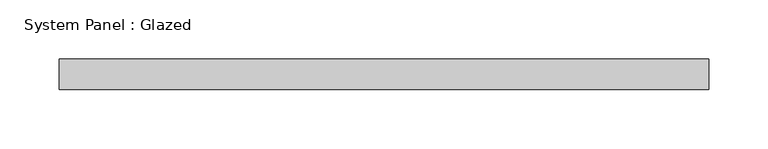
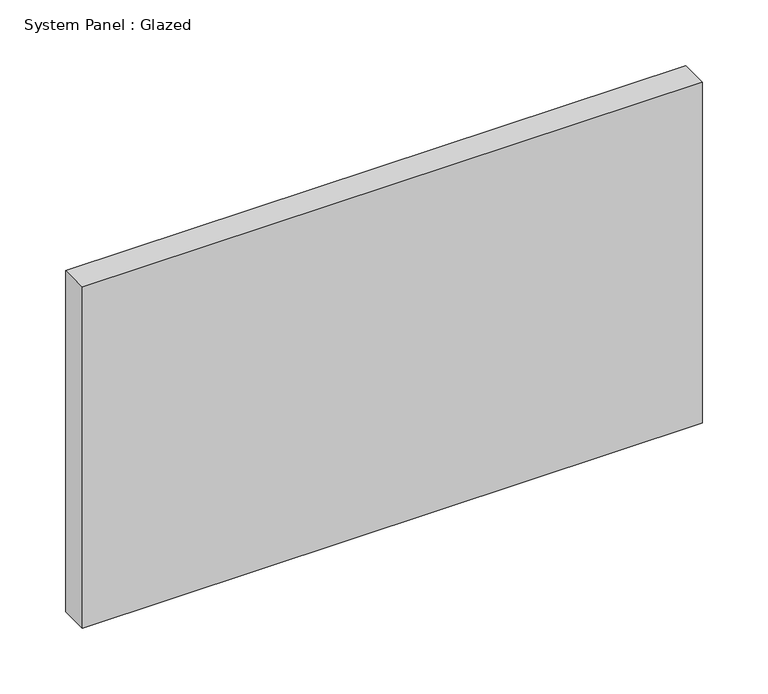
"""IFC4 building model written with IfcOpenShell, lengths in millimetres: plate geometry, System Panel : Glazed."""

from ifc_helpers import new_model, si_unit, origin, origin_with_axes, place, context, project, spatial, polyline, outline, extrude, source, transform, mapped, element, save


def system_panel_glazed_f12bf2b5(model_context):
    return source(origin(), model_context, "Body", "SweptSolid", [
        extrude(outline(polyline([(273.05, 19.05), (-273.05, 19.05), (-273.05, 44.45), (273.05, 44.45), (273.05, 19.05)])), origin_with_axes(), (0.0, 0.0, 1.0), 317.5),
    ])


if __name__ == "__main__":
    model = new_model("IFC4")
    model_context = context("Model", 3, world=origin())
    ifc_project = project(units=[si_unit("LENGTHUNIT", "METRE", prefix="MILLI")], contexts=[model_context])
    site = spatial("IfcSite", under=ifc_project)
    building = spatial("IfcBuilding", under=site)
    placement = place(None, origin())
    system_panel_glazed_shape = system_panel_glazed_f12bf2b5(model_context)
    element("IfcPlate", 1, ObjectType="System Panel : Glazed", at=placement, inside=building, context=model_context, shape_type="MappedRepresentation", body=[
        mapped(system_panel_glazed_shape, transform((0.0, 0.0, 0.0), x_axis=(1.0, 0.0, 0.0), y_axis=(0.0, 1.0, 0.0), z_axis=(0.0, 0.0, 1.0))),
    ])
    save(model, "model.ifc")

# Revit data of these elements
# Type "System Panel : Glazed"
#   Construction Type Id = "GSP4R"
#   Analytic Construction = "1/8 in Pilkington single glazing"
#   Visual Light Transmittance = 0.9
#   Solar Heat Gain Coefficient = 0.86
#   Heat Transfer Coefficient (U) = 1.18115 BTU/(h·ft²·°F)
#   Define Thermal Properties by = 1
# Element 1 (IfcPlate, "System Panel : Glazed")
#   Materials on its faces: "Glass"
# Materials
#   "Glass": class "Glass", colour RGB 0 128 192, transparency 0.75, Description = "Soda Lime Glass", Cost = 0
